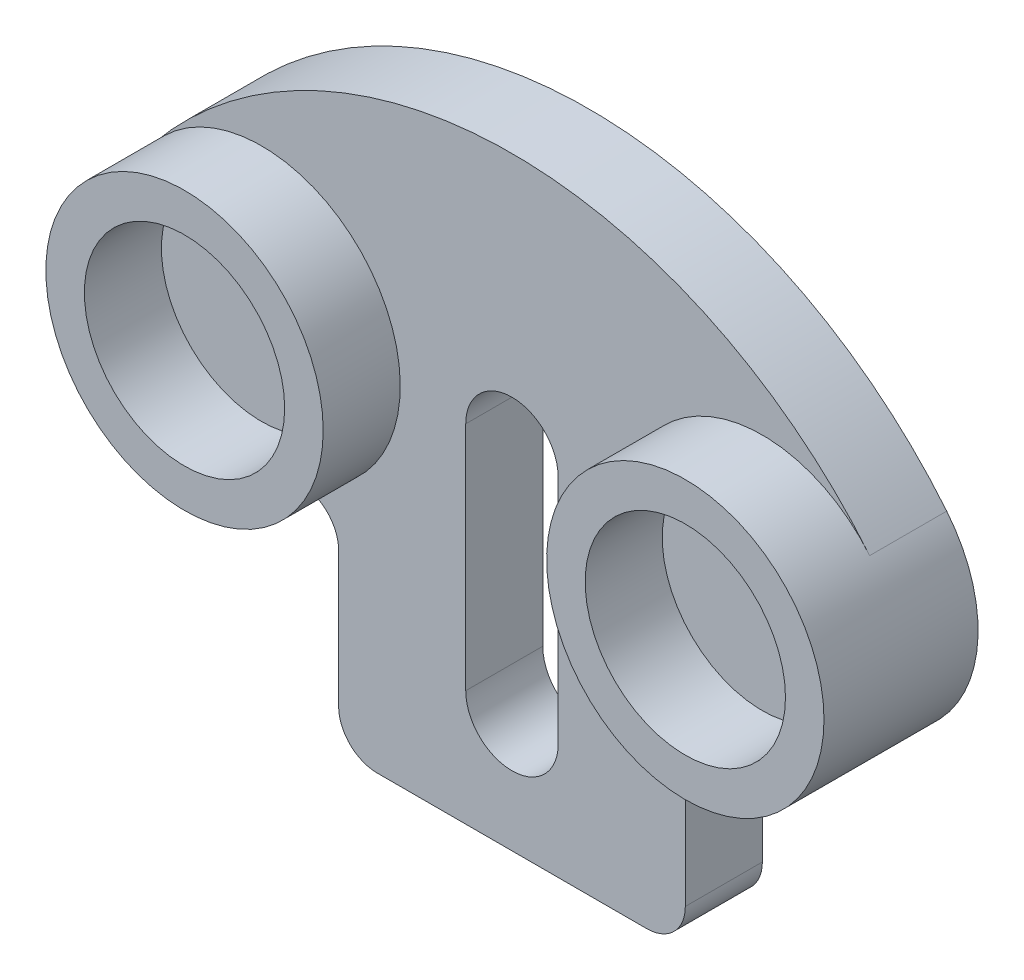
ISO-10303-21;
HEADER;
FILE_DESCRIPTION(('STEP AP214'),'2;1');
FILE_NAME('part.step','',(''),(''),'','','');
FILE_SCHEMA(('AUTOMOTIVE_DESIGN { 1 0 10303 214 1 1 1 1 }'));
ENDSEC;
DATA;
#1=APPLICATION_CONTEXT('core data for automotive mechanical design processes');
#2=APPLICATION_PROTOCOL_DEFINITION('international standard','automotive_design',2000,#1);
#3=PRODUCT_CONTEXT('',#1,'mechanical');
#4=PRODUCT('Part','Part','',(#3));
#5=PRODUCT_RELATED_PRODUCT_CATEGORY('part','',(#4));
#6=PRODUCT_DEFINITION_FORMATION('','',#4);
#7=PRODUCT_DEFINITION_CONTEXT('part definition',#1,'design');
#8=PRODUCT_DEFINITION('design','',#6,#7);
#9=PRODUCT_DEFINITION_SHAPE('','',#8);
#10=(LENGTH_UNIT() NAMED_UNIT(*) SI_UNIT(.MILLI.,.METRE.));
#11=(NAMED_UNIT(*) PLANE_ANGLE_UNIT() SI_UNIT($,.RADIAN.));
#12=(NAMED_UNIT(*) SI_UNIT($,.STERADIAN.) SOLID_ANGLE_UNIT());
#13=UNCERTAINTY_MEASURE_WITH_UNIT(LENGTH_MEASURE(1.E-05),#10,'distance_accuracy_value','');
#14=(GEOMETRIC_REPRESENTATION_CONTEXT(3) GLOBAL_UNCERTAINTY_ASSIGNED_CONTEXT((#13)) GLOBAL_UNIT_ASSIGNED_CONTEXT((#10,
#11,#12)) REPRESENTATION_CONTEXT('',''));
#15=CARTESIAN_POINT('',(0.,0.,0.));
#16=DIRECTION('',(0.,0.,1.));
#17=DIRECTION('',(1.,0.,0.));
#18=AXIS2_PLACEMENT_3D('',#15,#16,#17);
#19=CARTESIAN_POINT('',(0.,0.,10.));
#20=DIRECTION('',(0.,0.,1.));
#21=DIRECTION('',(1.,0.,0.));
#22=AXIS2_PLACEMENT_3D('',#19,#20,#21);
#23=PLANE('',#22);
#24=DIRECTION('',(0.,-1.,0.));
#25=VECTOR('',#24,1.);
#26=CARTESIAN_POINT('',(26.5,0.,10.));
#27=LINE('',#26,#25);
#28=CARTESIAN_POINT('',(26.5,0.,10.));
#29=VERTEX_POINT('',#28);
#30=CARTESIAN_POINT('',(26.5,-30.,10.));
#31=VERTEX_POINT('',#30);
#32=EDGE_CURVE('E58',#29,#31,#27,.T.);
#33=ORIENTED_EDGE('',*,*,#32,.F.);
#34=CARTESIAN_POINT('',(32.5,0.,10.));
#35=DIRECTION('',(0.,0.,1.));
#36=DIRECTION('',(1.,0.,0.));
#37=AXIS2_PLACEMENT_3D('',#34,#35,#36);
#38=CIRCLE('',#37,6.);
#39=CARTESIAN_POINT('',(38.5,0.,10.));
#40=VERTEX_POINT('',#39);
#41=EDGE_CURVE('E163',#40,#29,#38,.T.);
#42=ORIENTED_EDGE('',*,*,#41,.F.);
#43=DIRECTION('',(0.,-1.,0.));
#44=VECTOR('',#43,1.);
#45=CARTESIAN_POINT('',(38.5,0.,10.));
#46=LINE('',#45,#44);
#47=CARTESIAN_POINT('',(38.5,-30.,10.));
#48=VERTEX_POINT('',#47);
#49=EDGE_CURVE('E149',#40,#48,#46,.T.);
#50=ORIENTED_EDGE('',*,*,#49,.T.);
#51=CARTESIAN_POINT('',(32.5,-30.,10.));
#52=DIRECTION('',(0.,0.,1.));
#53=DIRECTION('',(1.,0.,0.));
#54=AXIS2_PLACEMENT_3D('',#51,#52,#53);
#55=CIRCLE('',#54,6.);
#56=EDGE_CURVE('E158',#31,#48,#55,.T.);
#57=ORIENTED_EDGE('',*,*,#56,.F.);
#58=EDGE_LOOP('',(#33,#42,#50,#57));
#59=FACE_BOUND('',#58,.T.);
#60=CARTESIAN_POINT('',(60.,-22.4499443206436,10.));
#61=DIRECTION('',(0.,0.,1.));
#62=DIRECTION('',(1.,0.,0.));
#63=AXIS2_PLACEMENT_3D('',#60,#61,#62);
#64=CIRCLE('',#63,5.);
#65=CARTESIAN_POINT('',(55.,-22.4499443206436,10.));
#66=VERTEX_POINT('',#65);
#67=CARTESIAN_POINT('',(61.0869565217391,-17.5695216422429,10.));
#68=VERTEX_POINT('',#67);
#69=EDGE_CURVE('E208',#66,#68,#64,.F.);
#70=ORIENTED_EDGE('',*,*,#69,.T.);
#71=CARTESIAN_POINT('',(65.,0.,10.));
#72=DIRECTION('',(0.,0.,1.));
#73=DIRECTION('',(1.,0.,0.));
#74=AXIS2_PLACEMENT_3D('',#71,#72,#73);
#75=CIRCLE('',#74,18.);
#76=CARTESIAN_POINT('',(78.9285714285714,11.4015305095054,10.));
#77=VERTEX_POINT('',#76);
#78=EDGE_CURVE('E180',#77,#68,#75,.T.);
#79=ORIENTED_EDGE('',*,*,#78,.F.);
#80=CARTESIAN_POINT('',(32.5,-26.603571188846,10.));
#81=DIRECTION('',(0.,0.,1.));
#82=DIRECTION('',(1.,0.,0.));
#83=AXIS2_PLACEMENT_3D('',#80,#81,#82);
#84=CIRCLE('',#83,60.);
#85=CARTESIAN_POINT('',(-13.9285714285714,11.4015305095055,10.));
#86=VERTEX_POINT('',#85);
#87=EDGE_CURVE('E209',#86,#77,#84,.F.);
#88=ORIENTED_EDGE('',*,*,#87,.F.);
#89=CARTESIAN_POINT('',(0.,0.,10.));
#90=DIRECTION('',(0.,0.,1.));
#91=DIRECTION('',(1.,0.,0.));
#92=AXIS2_PLACEMENT_3D('',#89,#90,#91);
#93=CIRCLE('',#92,18.);
#94=CARTESIAN_POINT('',(3.91304347826086,-17.5695216422429,10.));
#95=VERTEX_POINT('',#94);
#96=EDGE_CURVE('E192',#95,#86,#93,.T.);
#97=ORIENTED_EDGE('',*,*,#96,.F.);
#98=CARTESIAN_POINT('',(4.99999999999999,-22.4499443206436,10.));
#99=DIRECTION('',(0.,0.,1.));
#100=DIRECTION('',(1.,0.,0.));
#101=AXIS2_PLACEMENT_3D('',#98,#99,#100);
#102=CIRCLE('',#101,5.);
#103=CARTESIAN_POINT('',(9.99999999999999,-22.4499443206436,10.));
#104=VERTEX_POINT('',#103);
#105=EDGE_CURVE('E215',#104,#95,#102,.T.);
#106=ORIENTED_EDGE('',*,*,#105,.F.);
#107=DIRECTION('',(0.,1.,0.));
#108=VECTOR('',#107,1.);
#109=CARTESIAN_POINT('',(10.,0.,10.));
#110=LINE('',#109,#108);
#111=CARTESIAN_POINT('',(9.99999999999999,-40.,10.));
#112=VERTEX_POINT('',#111);
#113=EDGE_CURVE('E214',#112,#104,#110,.T.);
#114=ORIENTED_EDGE('',*,*,#113,.F.);
#115=CARTESIAN_POINT('',(15.,-40.,10.));
#116=DIRECTION('',(0.,0.,1.));
#117=DIRECTION('',(1.,0.,0.));
#118=AXIS2_PLACEMENT_3D('',#115,#116,#117);
#119=CIRCLE('',#118,5.);
#120=CARTESIAN_POINT('',(15.,-45.,10.));
#121=VERTEX_POINT('',#120);
#122=EDGE_CURVE('E217',#121,#112,#119,.F.);
#123=ORIENTED_EDGE('',*,*,#122,.F.);
#124=DIRECTION('',(1.,0.,0.));
#125=VECTOR('',#124,1.);
#126=CARTESIAN_POINT('',(0.,-45.,10.));
#127=LINE('',#126,#125);
#128=CARTESIAN_POINT('',(50.,-45.,10.));
#129=VERTEX_POINT('',#128);
#130=EDGE_CURVE('E199',#121,#129,#127,.T.);
#131=ORIENTED_EDGE('',*,*,#130,.T.);
#132=CARTESIAN_POINT('',(50.,-40.,10.));
#133=DIRECTION('',(0.,0.,1.));
#134=DIRECTION('',(1.,0.,0.));
#135=AXIS2_PLACEMENT_3D('',#132,#133,#134);
#136=CIRCLE('',#135,5.);
#137=CARTESIAN_POINT('',(55.,-40.,10.));
#138=VERTEX_POINT('',#137);
#139=EDGE_CURVE('E201',#129,#138,#136,.T.);
#140=ORIENTED_EDGE('',*,*,#139,.T.);
#141=DIRECTION('',(0.,1.,0.));
#142=VECTOR('',#141,1.);
#143=CARTESIAN_POINT('',(55.,0.,10.));
#144=LINE('',#143,#142);
#145=EDGE_CURVE('E206',#138,#66,#144,.T.);
#146=ORIENTED_EDGE('',*,*,#145,.T.);
#147=EDGE_LOOP('',(#70,#79,#88,#97,#106,#114,#123,#131,#140,#146));
#148=FACE_BOUND('',#147,.T.);
#149=ADVANCED_FACE('F44',(#59,#148),#23,.T.);
#150=CARTESIAN_POINT('',(0.,-45.,10.));
#151=DIRECTION('',(0.,1.,0.));
#152=DIRECTION('',(0.,0.,1.));
#153=AXIS2_PLACEMENT_3D('',#150,#151,#152);
#154=PLANE('',#153);
#155=DIRECTION('',(1.,0.,0.));
#156=VECTOR('',#155,1.);
#157=CARTESIAN_POINT('',(0.,-45.,0.));
#158=LINE('',#157,#156);
#159=CARTESIAN_POINT('',(15.,-45.,0.));
#160=VERTEX_POINT('',#159);
#161=CARTESIAN_POINT('',(50.,-45.,0.));
#162=VERTEX_POINT('',#161);
#163=EDGE_CURVE('E194',#160,#162,#158,.T.);
#164=ORIENTED_EDGE('',*,*,#163,.T.);
#165=DIRECTION('',(0.,0.,-1.));
#166=VECTOR('',#165,1.);
#167=CARTESIAN_POINT('',(50.,-45.,10.));
#168=LINE('',#167,#166);
#169=EDGE_CURVE('E200',#129,#162,#168,.T.);
#170=ORIENTED_EDGE('',*,*,#169,.F.);
#171=ORIENTED_EDGE('',*,*,#130,.F.);
#172=DIRECTION('',(0.,0.,-1.));
#173=VECTOR('',#172,1.);
#174=CARTESIAN_POINT('',(15.,-45.,10.));
#175=LINE('',#174,#173);
#176=EDGE_CURVE('E222',#121,#160,#175,.T.);
#177=ORIENTED_EDGE('',*,*,#176,.T.);
#178=EDGE_LOOP('',(#164,#170,#171,#177));
#179=FACE_BOUND('',#178,.T.);
#180=ADVANCED_FACE('F50',(#179),#154,.F.);
#181=CARTESIAN_POINT('',(50.,-40.,10.));
#182=DIRECTION('',(0.,0.,-1.));
#183=DIRECTION('',(-1.,0.,0.));
#184=AXIS2_PLACEMENT_3D('',#181,#182,#183);
#185=CYLINDRICAL_SURFACE('',#184,5.);
#186=CARTESIAN_POINT('',(50.,-40.,0.));
#187=DIRECTION('',(0.,0.,1.));
#188=DIRECTION('',(1.,0.,0.));
#189=AXIS2_PLACEMENT_3D('',#186,#187,#188);
#190=CIRCLE('',#189,5.);
#191=CARTESIAN_POINT('',(55.,-40.,0.));
#192=VERTEX_POINT('',#191);
#193=EDGE_CURVE('E221',#162,#192,#190,.T.);
#194=ORIENTED_EDGE('',*,*,#193,.T.);
#195=DIRECTION('',(0.,0.,-1.));
#196=VECTOR('',#195,1.);
#197=CARTESIAN_POINT('',(55.,-40.,10.));
#198=LINE('',#197,#196);
#199=EDGE_CURVE('E262',#138,#192,#198,.T.);
#200=ORIENTED_EDGE('',*,*,#199,.F.);
#201=ORIENTED_EDGE('',*,*,#139,.F.);
#202=ORIENTED_EDGE('',*,*,#169,.T.);
#203=EDGE_LOOP('',(#194,#200,#201,#202));
#204=FACE_BOUND('',#203,.T.);
#205=ADVANCED_FACE('F293',(#204),#185,.T.);
#206=CARTESIAN_POINT('',(55.,0.,10.));
#207=DIRECTION('',(-1.,0.,0.));
#208=DIRECTION('',(0.,-1.,0.));
#209=AXIS2_PLACEMENT_3D('',#206,#207,#208);
#210=PLANE('',#209);
#211=DIRECTION('',(0.,1.,0.));
#212=VECTOR('',#211,1.);
#213=CARTESIAN_POINT('',(55.,0.,0.));
#214=LINE('',#213,#212);
#215=CARTESIAN_POINT('',(55.,-22.4499443206436,0.));
#216=VERTEX_POINT('',#215);
#217=EDGE_CURVE('E229',#192,#216,#214,.T.);
#218=ORIENTED_EDGE('',*,*,#217,.T.);
#219=DIRECTION('',(0.,0.,-1.));
#220=VECTOR('',#219,1.);
#221=CARTESIAN_POINT('',(55.,-22.4499443206436,10.));
#222=LINE('',#221,#220);
#223=EDGE_CURVE('E261',#66,#216,#222,.T.);
#224=ORIENTED_EDGE('',*,*,#223,.F.);
#225=ORIENTED_EDGE('',*,*,#145,.F.);
#226=ORIENTED_EDGE('',*,*,#199,.T.);
#227=EDGE_LOOP('',(#218,#224,#225,#226));
#228=FACE_BOUND('',#227,.T.);
#229=ADVANCED_FACE('F329',(#228),#210,.F.);
#230=CARTESIAN_POINT('',(60.,-22.4499443206436,10.));
#231=DIRECTION('',(0.,0.,-1.));
#232=DIRECTION('',(-1.,0.,0.));
#233=AXIS2_PLACEMENT_3D('',#230,#231,#232);
#234=CYLINDRICAL_SURFACE('',#233,5.);
#235=CARTESIAN_POINT('',(60.,-22.4499443206436,0.));
#236=DIRECTION('',(0.,0.,1.));
#237=DIRECTION('',(1.,0.,0.));
#238=AXIS2_PLACEMENT_3D('',#235,#236,#237);
#239=CIRCLE('',#238,5.);
#240=CARTESIAN_POINT('',(61.0869565217391,-17.5695216422429,0.));
#241=VERTEX_POINT('',#240);
#242=EDGE_CURVE('E230',#216,#241,#239,.F.);
#243=ORIENTED_EDGE('',*,*,#242,.T.);
#244=DIRECTION('',(0.,0.,-1.));
#245=VECTOR('',#244,1.);
#246=CARTESIAN_POINT('',(61.0869565217391,-17.5695216422429,10.));
#247=LINE('',#246,#245);
#248=EDGE_CURVE('E256',#68,#241,#247,.T.);
#249=ORIENTED_EDGE('',*,*,#248,.F.);
#250=ORIENTED_EDGE('',*,*,#69,.F.);
#251=ORIENTED_EDGE('',*,*,#223,.T.);
#252=EDGE_LOOP('',(#243,#249,#250,#251));
#253=FACE_BOUND('',#252,.T.);
#254=ADVANCED_FACE('F326',(#253),#234,.F.);
#255=CARTESIAN_POINT('',(65.,0.,10.));
#256=DIRECTION('',(0.,0.,-1.));
#257=DIRECTION('',(-1.,0.,0.));
#258=AXIS2_PLACEMENT_3D('',#255,#256,#257);
#259=CYLINDRICAL_SURFACE('',#258,18.);
#260=CARTESIAN_POINT('',(65.,0.,0.));
#261=DIRECTION('',(0.,0.,1.));
#262=DIRECTION('',(1.,0.,0.));
#263=AXIS2_PLACEMENT_3D('',#260,#261,#262);
#264=CIRCLE('',#263,18.);
#265=CARTESIAN_POINT('',(78.9285714285714,11.4015305095054,0.));
#266=VERTEX_POINT('',#265);
#267=EDGE_CURVE('E227',#241,#266,#264,.T.);
#268=ORIENTED_EDGE('',*,*,#267,.T.);
#269=DIRECTION('',(0.,0.,-1.));
#270=VECTOR('',#269,1.);
#271=CARTESIAN_POINT('',(78.9285714285714,11.4015305095054,10.));
#272=LINE('',#271,#270);
#273=EDGE_CURVE('E258',#77,#266,#272,.T.);
#274=ORIENTED_EDGE('',*,*,#273,.F.);
#275=ORIENTED_EDGE('',*,*,#78,.T.);
#276=ORIENTED_EDGE('',*,*,#248,.T.);
#277=EDGE_LOOP('',(#268,#274,#275,#276));
#278=FACE_BOUND('',#277,.T.);
#279=CARTESIAN_POINT('',(65.,0.,20.));
#280=DIRECTION('',(0.,0.,1.));
#281=DIRECTION('',(1.,0.,0.));
#282=AXIS2_PLACEMENT_3D('',#279,#280,#281);
#283=CIRCLE('',#282,18.);
#284=CARTESIAN_POINT('',(83.,0.,20.));
#285=VERTEX_POINT('',#284);
#286=EDGE_CURVE('E189',#285,#285,#283,.T.);
#287=ORIENTED_EDGE('',*,*,#286,.F.);
#288=EDGE_LOOP('',(#287));
#289=FACE_BOUND('',#288,.T.);
#290=ADVANCED_FACE('F325',(#278,#289),#259,.T.);
#291=CARTESIAN_POINT('',(32.5,-26.603571188846,10.));
#292=DIRECTION('',(0.,0.,-1.));
#293=DIRECTION('',(-1.,0.,0.));
#294=AXIS2_PLACEMENT_3D('',#291,#292,#293);
#295=CYLINDRICAL_SURFACE('',#294,60.);
#296=CARTESIAN_POINT('',(32.5,-26.603571188846,0.));
#297=DIRECTION('',(0.,0.,1.));
#298=DIRECTION('',(1.,0.,0.));
#299=AXIS2_PLACEMENT_3D('',#296,#297,#298);
#300=CIRCLE('',#299,60.);
#301=CARTESIAN_POINT('',(-13.9285714285714,11.4015305095055,0.));
#302=VERTEX_POINT('',#301);
#303=EDGE_CURVE('E231',#302,#266,#300,.F.);
#304=ORIENTED_EDGE('',*,*,#303,.F.);
#305=DIRECTION('',(0.,0.,-1.));
#306=VECTOR('',#305,1.);
#307=CARTESIAN_POINT('',(-13.9285714285714,11.4015305095055,10.));
#308=LINE('',#307,#306);
#309=EDGE_CURVE('E255',#86,#302,#308,.T.);
#310=ORIENTED_EDGE('',*,*,#309,.F.);
#311=ORIENTED_EDGE('',*,*,#87,.T.);
#312=ORIENTED_EDGE('',*,*,#273,.T.);
#313=EDGE_LOOP('',(#304,#310,#311,#312));
#314=FACE_BOUND('',#313,.T.);
#315=ADVANCED_FACE('F318',(#314),#295,.T.);
#316=CARTESIAN_POINT('',(0.,0.,10.));
#317=DIRECTION('',(0.,0.,-1.));
#318=DIRECTION('',(-1.,0.,0.));
#319=AXIS2_PLACEMENT_3D('',#316,#317,#318);
#320=CYLINDRICAL_SURFACE('',#319,18.);
#321=CARTESIAN_POINT('',(0.,0.,0.));
#322=DIRECTION('',(0.,0.,1.));
#323=DIRECTION('',(1.,0.,0.));
#324=AXIS2_PLACEMENT_3D('',#321,#322,#323);
#325=CIRCLE('',#324,18.);
#326=CARTESIAN_POINT('',(3.91304347826086,-17.5695216422429,0.));
#327=VERTEX_POINT('',#326);
#328=EDGE_CURVE('E237',#302,#327,#325,.T.);
#329=ORIENTED_EDGE('',*,*,#328,.T.);
#330=DIRECTION('',(0.,0.,-1.));
#331=VECTOR('',#330,1.);
#332=CARTESIAN_POINT('',(3.91304347826086,-17.5695216422429,10.));
#333=LINE('',#332,#331);
#334=EDGE_CURVE('E252',#95,#327,#333,.T.);
#335=ORIENTED_EDGE('',*,*,#334,.F.);
#336=ORIENTED_EDGE('',*,*,#96,.T.);
#337=ORIENTED_EDGE('',*,*,#309,.T.);
#338=EDGE_LOOP('',(#329,#335,#336,#337));
#339=FACE_BOUND('',#338,.T.);
#340=CARTESIAN_POINT('',(0.,0.,20.));
#341=DIRECTION('',(0.,0.,1.));
#342=DIRECTION('',(1.,0.,0.));
#343=AXIS2_PLACEMENT_3D('',#340,#341,#342);
#344=CIRCLE('',#343,18.);
#345=CARTESIAN_POINT('',(18.,0.,20.));
#346=VERTEX_POINT('',#345);
#347=EDGE_CURVE('E188',#346,#346,#344,.T.);
#348=ORIENTED_EDGE('',*,*,#347,.F.);
#349=EDGE_LOOP('',(#348));
#350=FACE_BOUND('',#349,.T.);
#351=ADVANCED_FACE('F314',(#339,#350),#320,.T.);
#352=CARTESIAN_POINT('',(4.99999999999999,-22.4499443206436,10.));
#353=DIRECTION('',(0.,0.,-1.));
#354=DIRECTION('',(-1.,0.,0.));
#355=AXIS2_PLACEMENT_3D('',#352,#353,#354);
#356=CYLINDRICAL_SURFACE('',#355,5.);
#357=CARTESIAN_POINT('',(4.99999999999999,-22.4499443206436,0.));
#358=DIRECTION('',(0.,0.,1.));
#359=DIRECTION('',(1.,0.,0.));
#360=AXIS2_PLACEMENT_3D('',#357,#358,#359);
#361=CIRCLE('',#360,5.);
#362=CARTESIAN_POINT('',(9.99999999999999,-22.4499443206436,0.));
#363=VERTEX_POINT('',#362);
#364=EDGE_CURVE('E239',#363,#327,#361,.T.);
#365=ORIENTED_EDGE('',*,*,#364,.F.);
#366=DIRECTION('',(0.,0.,-1.));
#367=VECTOR('',#366,1.);
#368=CARTESIAN_POINT('',(9.99999999999999,-22.4499443206436,10.));
#369=LINE('',#368,#367);
#370=EDGE_CURVE('E247',#104,#363,#369,.T.);
#371=ORIENTED_EDGE('',*,*,#370,.F.);
#372=ORIENTED_EDGE('',*,*,#105,.T.);
#373=ORIENTED_EDGE('',*,*,#334,.T.);
#374=EDGE_LOOP('',(#365,#371,#372,#373));
#375=FACE_BOUND('',#374,.T.);
#376=ADVANCED_FACE('F309',(#375),#356,.F.);
#377=CARTESIAN_POINT('',(10.,0.,10.));
#378=DIRECTION('',(-1.,0.,0.));
#379=DIRECTION('',(0.,-1.,0.));
#380=AXIS2_PLACEMENT_3D('',#377,#378,#379);
#381=PLANE('',#380);
#382=DIRECTION('',(0.,1.,0.));
#383=VECTOR('',#382,1.);
#384=CARTESIAN_POINT('',(10.,0.,0.));
#385=LINE('',#384,#383);
#386=CARTESIAN_POINT('',(9.99999999999999,-40.,0.));
#387=VERTEX_POINT('',#386);
#388=EDGE_CURVE('E241',#387,#363,#385,.T.);
#389=ORIENTED_EDGE('',*,*,#388,.F.);
#390=DIRECTION('',(0.,0.,-1.));
#391=VECTOR('',#390,1.);
#392=CARTESIAN_POINT('',(9.99999999999999,-40.,10.));
#393=LINE('',#392,#391);
#394=EDGE_CURVE('E246',#112,#387,#393,.T.);
#395=ORIENTED_EDGE('',*,*,#394,.F.);
#396=ORIENTED_EDGE('',*,*,#113,.T.);
#397=ORIENTED_EDGE('',*,*,#370,.T.);
#398=EDGE_LOOP('',(#389,#395,#396,#397));
#399=FACE_BOUND('',#398,.T.);
#400=ADVANCED_FACE('F308',(#399),#381,.T.);
#401=CARTESIAN_POINT('',(15.,-40.,10.));
#402=DIRECTION('',(0.,0.,-1.));
#403=DIRECTION('',(-1.,0.,0.));
#404=AXIS2_PLACEMENT_3D('',#401,#402,#403);
#405=CYLINDRICAL_SURFACE('',#404,5.);
#406=CARTESIAN_POINT('',(15.,-40.,0.));
#407=DIRECTION('',(0.,0.,1.));
#408=DIRECTION('',(1.,0.,0.));
#409=AXIS2_PLACEMENT_3D('',#406,#407,#408);
#410=CIRCLE('',#409,5.);
#411=EDGE_CURVE('E204',#160,#387,#410,.F.);
#412=ORIENTED_EDGE('',*,*,#411,.F.);
#413=ORIENTED_EDGE('',*,*,#176,.F.);
#414=ORIENTED_EDGE('',*,*,#122,.T.);
#415=ORIENTED_EDGE('',*,*,#394,.T.);
#416=EDGE_LOOP('',(#412,#413,#414,#415));
#417=FACE_BOUND('',#416,.T.);
#418=ADVANCED_FACE('F301',(#417),#405,.T.);
#419=CARTESIAN_POINT('',(0.,0.,0.));
#420=DIRECTION('',(0.,0.,1.));
#421=DIRECTION('',(1.,0.,0.));
#422=AXIS2_PLACEMENT_3D('',#419,#420,#421);
#423=PLANE('',#422);
#424=CARTESIAN_POINT('',(32.5,0.,0.));
#425=DIRECTION('',(0.,0.,1.));
#426=DIRECTION('',(1.,0.,0.));
#427=AXIS2_PLACEMENT_3D('',#424,#425,#426);
#428=CIRCLE('',#427,6.);
#429=CARTESIAN_POINT('',(38.5,0.,0.));
#430=VERTEX_POINT('',#429);
#431=CARTESIAN_POINT('',(26.5,0.,0.));
#432=VERTEX_POINT('',#431);
#433=EDGE_CURVE('E52',#430,#432,#428,.T.);
#434=ORIENTED_EDGE('',*,*,#433,.T.);
#435=DIRECTION('',(0.,-1.,0.));
#436=VECTOR('',#435,1.);
#437=CARTESIAN_POINT('',(26.5,0.,0.));
#438=LINE('',#437,#436);
#439=CARTESIAN_POINT('',(26.5,-30.,0.));
#440=VERTEX_POINT('',#439);
#441=EDGE_CURVE('E11',#432,#440,#438,.T.);
#442=ORIENTED_EDGE('',*,*,#441,.T.);
#443=CARTESIAN_POINT('',(32.5,-30.,0.));
#444=DIRECTION('',(0.,0.,1.));
#445=DIRECTION('',(1.,0.,0.));
#446=AXIS2_PLACEMENT_3D('',#443,#444,#445);
#447=CIRCLE('',#446,6.);
#448=CARTESIAN_POINT('',(38.5,-30.,0.));
#449=VERTEX_POINT('',#448);
#450=EDGE_CURVE('E196',#440,#449,#447,.T.);
#451=ORIENTED_EDGE('',*,*,#450,.T.);
#452=DIRECTION('',(0.,-1.,0.));
#453=VECTOR('',#452,1.);
#454=CARTESIAN_POINT('',(38.5,0.,0.));
#455=LINE('',#454,#453);
#456=EDGE_CURVE('E155',#430,#449,#455,.T.);
#457=ORIENTED_EDGE('',*,*,#456,.F.);
#458=EDGE_LOOP('',(#434,#442,#451,#457));
#459=FACE_BOUND('',#458,.T.);
#460=ORIENTED_EDGE('',*,*,#163,.F.);
#461=ORIENTED_EDGE('',*,*,#411,.T.);
#462=ORIENTED_EDGE('',*,*,#388,.T.);
#463=ORIENTED_EDGE('',*,*,#364,.T.);
#464=ORIENTED_EDGE('',*,*,#328,.F.);
#465=ORIENTED_EDGE('',*,*,#303,.T.);
#466=ORIENTED_EDGE('',*,*,#267,.F.);
#467=ORIENTED_EDGE('',*,*,#242,.F.);
#468=ORIENTED_EDGE('',*,*,#217,.F.);
#469=ORIENTED_EDGE('',*,*,#193,.F.);
#470=EDGE_LOOP('',(#460,#461,#462,#463,#464,#465,#466,#467,#468,#469));
#471=FACE_BOUND('',#470,.T.);
#472=ADVANCED_FACE('F275',(#459,#471),#423,.F.);
#473=CARTESIAN_POINT('',(0.,0.,20.));
#474=DIRECTION('',(0.,0.,1.));
#475=DIRECTION('',(1.,0.,0.));
#476=AXIS2_PLACEMENT_3D('',#473,#474,#475);
#477=PLANE('',#476);
#478=CARTESIAN_POINT('',(0.,0.,20.));
#479=DIRECTION('',(0.,0.,1.));
#480=DIRECTION('',(1.,0.,0.));
#481=AXIS2_PLACEMENT_3D('',#478,#479,#480);
#482=CIRCLE('',#481,13.);
#483=CARTESIAN_POINT('',(13.,0.,20.));
#484=VERTEX_POINT('',#483);
#485=EDGE_CURVE('E176',#484,#484,#482,.T.);
#486=ORIENTED_EDGE('',*,*,#485,.F.);
#487=EDGE_LOOP('',(#486));
#488=FACE_BOUND('',#487,.T.);
#489=ORIENTED_EDGE('',*,*,#347,.T.);
#490=EDGE_LOOP('',(#489));
#491=FACE_BOUND('',#490,.T.);
#492=ADVANCED_FACE('F298',(#488,#491),#477,.T.);
#493=CARTESIAN_POINT('',(65.,0.,20.));
#494=DIRECTION('',(0.,0.,1.));
#495=DIRECTION('',(1.,0.,0.));
#496=AXIS2_PLACEMENT_3D('',#493,#494,#495);
#497=PLANE('',#496);
#498=CARTESIAN_POINT('',(65.,0.,20.));
#499=DIRECTION('',(0.,0.,1.));
#500=DIRECTION('',(1.,0.,0.));
#501=AXIS2_PLACEMENT_3D('',#498,#499,#500);
#502=CIRCLE('',#501,13.);
#503=CARTESIAN_POINT('',(78.,0.,20.));
#504=VERTEX_POINT('',#503);
#505=EDGE_CURVE('E174',#504,#504,#502,.T.);
#506=ORIENTED_EDGE('',*,*,#505,.F.);
#507=EDGE_LOOP('',(#506));
#508=FACE_BOUND('',#507,.T.);
#509=ORIENTED_EDGE('',*,*,#286,.T.);
#510=EDGE_LOOP('',(#509));
#511=FACE_BOUND('',#510,.T.);
#512=ADVANCED_FACE('F368',(#508,#511),#497,.T.);
#513=CARTESIAN_POINT('',(65.,0.,10.));
#514=DIRECTION('',(0.,0.,1.));
#515=DIRECTION('',(1.,0.,0.));
#516=AXIS2_PLACEMENT_3D('',#513,#514,#515);
#517=CYLINDRICAL_SURFACE('',#516,13.);
#518=CARTESIAN_POINT('',(65.,0.,10.));
#519=DIRECTION('',(0.,0.,1.));
#520=DIRECTION('',(1.,0.,0.));
#521=AXIS2_PLACEMENT_3D('',#518,#519,#520);
#522=CIRCLE('',#521,13.);
#523=CARTESIAN_POINT('',(78.,0.,10.));
#524=VERTEX_POINT('',#523);
#525=EDGE_CURVE('E182',#524,#524,#522,.T.);
#526=ORIENTED_EDGE('',*,*,#525,.F.);
#527=EDGE_LOOP('',(#526));
#528=FACE_BOUND('',#527,.T.);
#529=ORIENTED_EDGE('',*,*,#505,.T.);
#530=EDGE_LOOP('',(#529));
#531=FACE_BOUND('',#530,.T.);
#532=ADVANCED_FACE('F371',(#528,#531),#517,.F.);
#533=CARTESIAN_POINT('',(65.,0.,10.));
#534=DIRECTION('',(0.,0.,1.));
#535=DIRECTION('',(1.,0.,0.));
#536=AXIS2_PLACEMENT_3D('',#533,#534,#535);
#537=PLANE('',#536);
#538=ORIENTED_EDGE('',*,*,#525,.T.);
#539=EDGE_LOOP('',(#538));
#540=FACE_BOUND('',#539,.T.);
#541=ADVANCED_FACE('F376',(#540),#537,.T.);
#542=CARTESIAN_POINT('',(0.,0.,10.));
#543=DIRECTION('',(0.,0.,1.));
#544=DIRECTION('',(1.,0.,0.));
#545=AXIS2_PLACEMENT_3D('',#542,#543,#544);
#546=CYLINDRICAL_SURFACE('',#545,13.);
#547=CARTESIAN_POINT('',(0.,0.,10.));
#548=DIRECTION('',(0.,0.,1.));
#549=DIRECTION('',(1.,0.,0.));
#550=AXIS2_PLACEMENT_3D('',#547,#548,#549);
#551=CIRCLE('',#550,13.);
#552=CARTESIAN_POINT('',(13.,0.,10.));
#553=VERTEX_POINT('',#552);
#554=EDGE_CURVE('E173',#553,#553,#551,.T.);
#555=ORIENTED_EDGE('',*,*,#554,.F.);
#556=EDGE_LOOP('',(#555));
#557=FACE_BOUND('',#556,.T.);
#558=ORIENTED_EDGE('',*,*,#485,.T.);
#559=EDGE_LOOP('',(#558));
#560=FACE_BOUND('',#559,.T.);
#561=ADVANCED_FACE('F288',(#557,#560),#546,.F.);
#562=CARTESIAN_POINT('',(0.,0.,10.));
#563=DIRECTION('',(0.,0.,1.));
#564=DIRECTION('',(1.,0.,0.));
#565=AXIS2_PLACEMENT_3D('',#562,#563,#564);
#566=PLANE('',#565);
#567=ORIENTED_EDGE('',*,*,#554,.T.);
#568=EDGE_LOOP('',(#567));
#569=FACE_BOUND('',#568,.T.);
#570=ADVANCED_FACE('F276',(#569),#566,.T.);
#571=CARTESIAN_POINT('',(26.5,0.,-10.));
#572=DIRECTION('',(-1.,0.,0.));
#573=DIRECTION('',(0.,0.,1.));
#574=AXIS2_PLACEMENT_3D('',#571,#572,#573);
#575=PLANE('',#574);
#576=DIRECTION('',(0.,0.,1.));
#577=VECTOR('',#576,1.);
#578=CARTESIAN_POINT('',(26.5,0.,-10.));
#579=LINE('',#578,#577);
#580=EDGE_CURVE('E166',#432,#29,#579,.T.);
#581=ORIENTED_EDGE('',*,*,#580,.T.);
#582=ORIENTED_EDGE('',*,*,#32,.T.);
#583=DIRECTION('',(0.,0.,1.));
#584=VECTOR('',#583,1.);
#585=CARTESIAN_POINT('',(26.5,-30.,-10.));
#586=LINE('',#585,#584);
#587=EDGE_CURVE('E154',#440,#31,#586,.T.);
#588=ORIENTED_EDGE('',*,*,#587,.F.);
#589=ORIENTED_EDGE('',*,*,#441,.F.);
#590=EDGE_LOOP('',(#581,#582,#588,#589));
#591=FACE_BOUND('',#590,.T.);
#592=ADVANCED_FACE('F280',(#591),#575,.F.);
#593=CARTESIAN_POINT('',(32.5,0.,-10.));
#594=DIRECTION('',(0.,0.,1.));
#595=DIRECTION('',(1.,0.,0.));
#596=AXIS2_PLACEMENT_3D('',#593,#594,#595);
#597=CYLINDRICAL_SURFACE('',#596,6.);
#598=DIRECTION('',(0.,0.,1.));
#599=VECTOR('',#598,1.);
#600=CARTESIAN_POINT('',(38.5,0.,-10.));
#601=LINE('',#600,#599);
#602=EDGE_CURVE('E152',#430,#40,#601,.T.);
#603=ORIENTED_EDGE('',*,*,#602,.T.);
#604=ORIENTED_EDGE('',*,*,#41,.T.);
#605=ORIENTED_EDGE('',*,*,#580,.F.);
#606=ORIENTED_EDGE('',*,*,#433,.F.);
#607=EDGE_LOOP('',(#603,#604,#605,#606));
#608=FACE_BOUND('',#607,.T.);
#609=ADVANCED_FACE('F277',(#608),#597,.F.);
#610=CARTESIAN_POINT('',(38.5,0.,-10.));
#611=DIRECTION('',(-1.,0.,0.));
#612=DIRECTION('',(0.,0.,1.));
#613=AXIS2_PLACEMENT_3D('',#610,#611,#612);
#614=PLANE('',#613);
#615=ORIENTED_EDGE('',*,*,#456,.T.);
#616=DIRECTION('',(0.,0.,1.));
#617=VECTOR('',#616,1.);
#618=CARTESIAN_POINT('',(38.5,-30.,-10.));
#619=LINE('',#618,#617);
#620=EDGE_CURVE('E66',#449,#48,#619,.T.);
#621=ORIENTED_EDGE('',*,*,#620,.T.);
#622=ORIENTED_EDGE('',*,*,#49,.F.);
#623=ORIENTED_EDGE('',*,*,#602,.F.);
#624=EDGE_LOOP('',(#615,#621,#622,#623));
#625=FACE_BOUND('',#624,.T.);
#626=ADVANCED_FACE('F148',(#625),#614,.T.);
#627=CARTESIAN_POINT('',(32.5,-30.,-10.));
#628=DIRECTION('',(0.,0.,1.));
#629=DIRECTION('',(1.,0.,0.));
#630=AXIS2_PLACEMENT_3D('',#627,#628,#629);
#631=CYLINDRICAL_SURFACE('',#630,6.);
#632=ORIENTED_EDGE('',*,*,#587,.T.);
#633=ORIENTED_EDGE('',*,*,#56,.T.);
#634=ORIENTED_EDGE('',*,*,#620,.F.);
#635=ORIENTED_EDGE('',*,*,#450,.F.);
#636=EDGE_LOOP('',(#632,#633,#634,#635));
#637=FACE_BOUND('',#636,.T.);
#638=ADVANCED_FACE('F157',(#637),#631,.F.);
#639=CLOSED_SHELL('',(#149,#180,#205,#229,#254,#290,#315,#351,#376,#400,#418,#472,#492,#512,
#532,#541,#561,#570,#592,#609,#626,#638));
#640=MANIFOLD_SOLID_BREP('B2',#639);
#641=ADVANCED_BREP_SHAPE_REPRESENTATION('',(#18,#640),#14);
#642=SHAPE_DEFINITION_REPRESENTATION(#9,#641);
ENDSEC;
END-ISO-10303-21;
